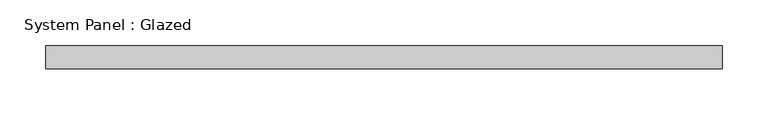
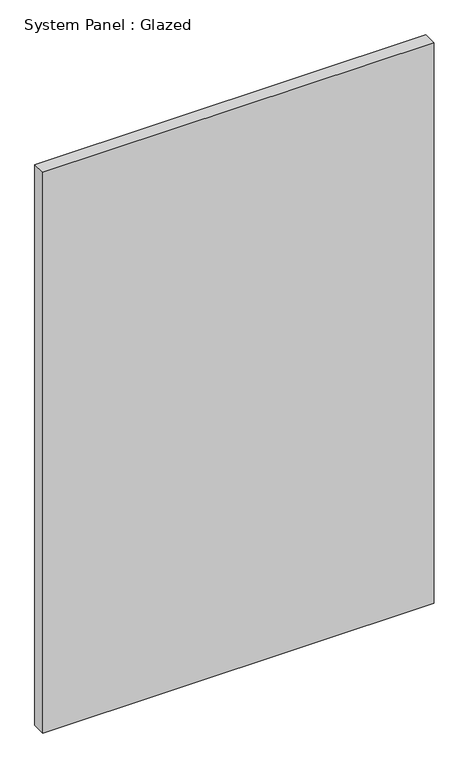
"""IFC4 building model written with IfcOpenShell, lengths in millimetres: plate geometry, System Panel : Glazed."""

from ifc_helpers import new_model, si_unit, origin, origin_with_axes, place, context, project, spatial, polyline, outline, extrude, source, transform, mapped, element, save


def system_panel_glazed_6160ed8e(model_context):
    return source(origin(), model_context, "Body", "SweptSolid", [
        extrude(outline(polyline([(370.4021, 19.05), (-370.4021, 19.05), (-370.4021, 44.45), (370.4021, 44.45), (370.4021, 19.05)])), origin_with_axes(), (0.0, 0.0, 1.0), 1121.8333333),
    ])


if __name__ == "__main__":
    model = new_model("IFC4")
    model_context = context("Model", 3, world=origin())
    ifc_project = project(units=[si_unit("LENGTHUNIT", "METRE", prefix="MILLI")], contexts=[model_context])
    site = spatial("IfcSite", under=ifc_project)
    building = spatial("IfcBuilding", under=site)
    placement = place(None, origin())
    system_panel_glazed_shape = system_panel_glazed_6160ed8e(model_context)
    element("IfcPlate", 1, ObjectType="System Panel : Glazed", at=placement, inside=building, context=model_context, shape_type="MappedRepresentation", body=[
        mapped(system_panel_glazed_shape, transform((0.0, 0.0, 0.0), x_axis=(1.0, 0.0, 0.0), y_axis=(0.0, 1.0, 0.0), z_axis=(0.0, 0.0, 1.0))),
    ])
    save(model, "model.ifc")

# Revit data of these elements
# Type "System Panel : Glazed"
#   Construction Type Id = "GSP4R"
#   Analytic Construction = "1/8 in Pilkington single glazing"
#   Visual Light Transmittance = 0.9
#   Solar Heat Gain Coefficient = 0.86
#   Heat Transfer Coefficient (U) = 1.18115 BTU/(h·ft²·°F)
#   Define Thermal Properties by = 1
# Element 1 (IfcPlate, "System Panel : Glazed")
#   Materials on its faces: "Glass"
# Materials
#   "Glass": class "Glass", colour RGB 0 128 192, transparency 0.75, Description = "Soda Lime Glass", Cost = 0
